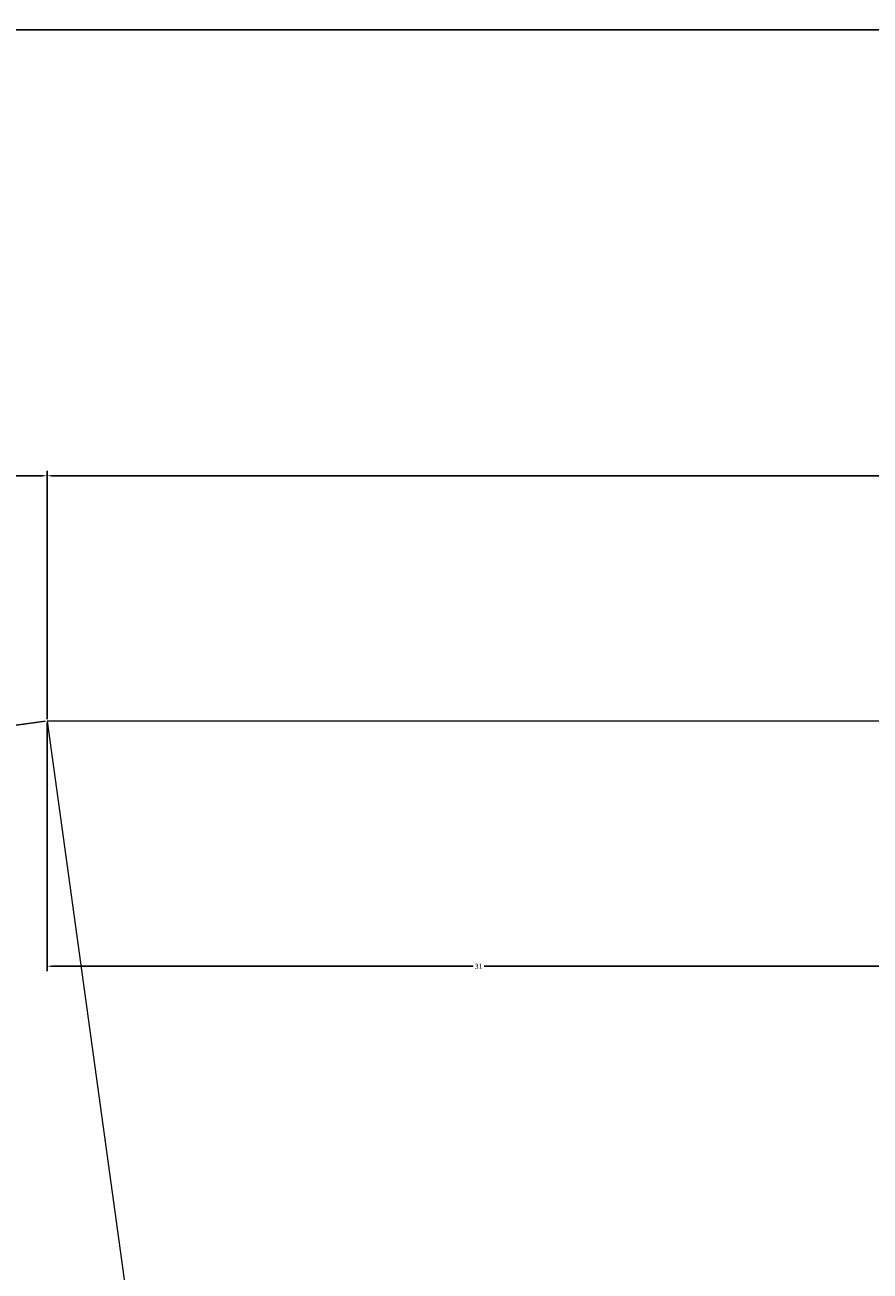
# Model space of a CAD drawing. Units: millimetres. Extents: x -9 to 135, y -119 to 27.
# Tile 5 of 12: x 31 to 62, y -18 to 27. Entities that reach past the tile are written whole.
import ezdxf

# ---------------------------------------------------------------- set-up
doc = ezdxf.new("R2010")
doc.units = ezdxf.units.MM
doc.layers.add('M-CONS', color=8, linetype='Continuous', lineweight=18)
doc.layers.add('M-DIMS', color=2, linetype='Continuous', lineweight=18)
doc.styles.get("Standard").update_dxf_attribs({"font": 'arial.ttf'})
doc.dimstyles.get("Standard").update_dxf_attribs({"dimtxt": 0.18, "dimasz": 0.18, "dimexe": 0.18, "dimexo": 0.0625, "dimgap": 0.09, "dimtad": 0, "dimtih": 1, "dimtoh": 1, "dimdec": 4, "dimzin": 0, "dimdsep": 46, "dimtxsty": 'Standard', "dimcen": 0.09, "dimadec": 0, "dimazin": 0, "dimtfac": 1, "dimtdec": 4, "dimtofl": 0, "dimtmove": 0, "dimatfit": 3, "dimfxl": 1, "dimtolj": 1, "dimtzin": 0, "dimarcsym": 0})

# ---------------------------------------------------------------- blocks, each defined once
blk = doc.blocks.new('*D2')
at = {"layer": 'Defpoints', "color": 0, "transparency": 16777216}
for p in [(126, 26.533), (0, 17.733), (126, 1.733)]:
    blk.add_point(p, dxfattribs=at)
at = {"layer": 'M-DIMS', "color": 0, "lineweight": -2, "transparency": 16777216}
for p, q in [((0, 17.796), (0, 26.713)), ((0.18, 26.533), (62.72, 26.533)), ((125.82, 26.533), (63.28, 26.533)), ((126, 1.796), (126, 26.713))]:
    blk.add_line(p, q, dxfattribs=at)
at = {"layer": 'M-DIMS', "color": 0, "transparency": 16777216}
for points in [[(0.18, 26.563), (0.18, 26.503), (0, 26.533)], [(125.82, 26.563), (125.82, 26.503), (126, 26.533)]]:
    blk.add_solid(points, dxfattribs=at)
at = {"layer": 'M-DIMS', "color": 0, "transparency": 16777216, "insert": (63, 26.533), "char_height": 0.18, "attachment_point": 5}
blk.add_mtext('\\A1;126', dxfattribs=at)
blk = doc.blocks.new('*D3')
at = {"layer": 'Defpoints', "color": 0, "transparency": 16777216}
for p in [(0, 17.733), (-8.8, -110.267), (63, -110.267)]:
    blk.add_point(p, dxfattribs=at)
at = {"layer": 'M-DIMS', "color": 0, "lineweight": -2, "transparency": 16777216}
for p, q in [((-0.062, 17.733), (-8.98, 17.733)), ((-8.8, 17.553), (-8.8, -46.085)), ((-8.8, -110.087), (-8.8, -46.449)), ((62.938, -110.267), (-8.98, -110.267))]:
    blk.add_line(p, q, dxfattribs=at)
at = {"layer": 'M-DIMS', "color": 0, "transparency": 16777216}
for points in [[(-8.83, 17.553), (-8.77, 17.553), (-8.8, 17.733)], [(-8.83, -110.087), (-8.77, -110.087), (-8.8, -110.267)]]:
    blk.add_solid(points, dxfattribs=at)
at = {"layer": 'M-DIMS', "color": 0, "transparency": 16777216, "insert": (-8.8, -46.267), "char_height": 0.18, "attachment_point": 5}
blk.add_mtext('\\A1;128', dxfattribs=at)
blk = doc.blocks.new('*D5')
at = {"layer": 'Defpoints', "color": 0, "transparency": 16777216}
for p in [(32, 10.533), (18, 1.733), (32, 1.733)]:
    blk.add_point(p, dxfattribs=at)
at = {"layer": 'M-DIMS', "color": 0, "lineweight": -2, "transparency": 16777216}
for p, q in [((18, 1.796), (18, 10.713)), ((18.18, 10.533), (24.79, 10.533)), ((31.82, 10.533), (25.21, 10.533)), ((32, 1.796), (32, 10.713))]:
    blk.add_line(p, q, dxfattribs=at)
at = {"layer": 'M-DIMS', "color": 0, "transparency": 16777216}
for points in [[(18.18, 10.563), (18.18, 10.503), (18, 10.533)], [(31.82, 10.563), (31.82, 10.503), (32, 10.533)]]:
    blk.add_solid(points, dxfattribs=at)
at = {"layer": 'M-DIMS', "color": 0, "transparency": 16777216, "insert": (25, 10.533), "char_height": 0.18, "attachment_point": 5}
blk.add_mtext('\\A1;14', dxfattribs=at)
blk = doc.blocks.new('*D6')
at = {"layer": 'Defpoints', "color": 0, "transparency": 16777216}
for p in [(94, 10.533), (32, 1.733), (94, 1.733)]:
    blk.add_point(p, dxfattribs=at)
at = {"layer": 'M-DIMS', "color": 0, "lineweight": -2, "transparency": 16777216}
for p, q in [((32, 1.796), (32, 10.713)), ((32.18, 10.533), (62.782, 10.533)), ((93.82, 10.533), (63.218, 10.533)), ((94, 1.796), (94, 10.713))]:
    blk.add_line(p, q, dxfattribs=at)
at = {"layer": 'M-DIMS', "color": 0, "transparency": 16777216}
for points in [[(32.18, 10.563), (32.18, 10.503), (32, 10.533)], [(93.82, 10.563), (93.82, 10.503), (94, 10.533)]]:
    blk.add_solid(points, dxfattribs=at)
at = {"layer": 'M-DIMS', "color": 0, "transparency": 16777216, "insert": (63, 10.533), "char_height": 0.18, "attachment_point": 5}
blk.add_mtext('\\A1;62', dxfattribs=at)
blk = doc.blocks.new('*D9')
at = {"layer": 'Defpoints', "color": 0, "transparency": 16777216}
for p in [(32, 1.733), (63, 1.733), (32, -7.067)]:
    blk.add_point(p, dxfattribs=at)
at = {"layer": 'M-DIMS', "color": 0, "lineweight": -2, "transparency": 16777216}
for p, q in [((32, 1.671), (32, -7.247)), ((63, 1.671), (63, -7.247)), ((32.18, -7.067), (47.299, -7.067)), ((62.82, -7.067), (47.701, -7.067))]:
    blk.add_line(p, q, dxfattribs=at)
at = {"layer": 'M-DIMS', "color": 0, "transparency": 16777216}
for points in [[(32.18, -7.037), (32.18, -7.097), (32, -7.067)], [(62.82, -7.037), (62.82, -7.097), (63, -7.067)]]:
    blk.add_solid(points, dxfattribs=at)
at = {"layer": 'M-DIMS', "color": 0, "transparency": 16777216, "insert": (47.5, -7.067), "char_height": 0.18, "attachment_point": 5}
blk.add_mtext('\\A1;31', dxfattribs=at)
blk = doc.blocks.new('*D14')
at = {"layer": 'Defpoints', "color": 0, "transparency": 16777216}
for p in [(32, 1.733), (23.283, 0.528), (45, -92.267)]:
    blk.add_point(p, dxfattribs=at)
at = {"layer": 'M-DIMS', "color": 0, "lineweight": -2, "transparency": 16777216}
for p, q in [((31.938, 1.725), (23.105, 0.503)), ((23.308, 0.349), (29.758, -46.29)), ((36.258, -93.294), (29.808, -46.654)), ((44.938, -92.275), (36.105, -93.497))]:
    blk.add_line(p, q, dxfattribs=at)
at = {"layer": 'M-DIMS', "color": 0, "transparency": 16777216}
for points in [[(23.337, 0.353), (23.278, 0.345), (23.283, 0.528)], [(36.288, -93.29), (36.229, -93.298), (36.283, -93.472)]]:
    blk.add_solid(points, dxfattribs=at)
at = {"layer": 'M-DIMS', "color": 0, "transparency": 16777216, "insert": (29.783, -46.472), "char_height": 0.18, "attachment_point": 5}
blk.add_mtext('\\A1;94.9', dxfattribs=at)

msp = doc.modelspace()

# ---------------------------------------------------------------- linework, layer by layer
at = {"layer": 'M-CONS'}
for p, q in [((63, 1.733, 115.129), (32, 1.733, 115.129)), ((32, 1.733, 115.129), (45, -92.267, 115.129))]:
    msp.add_line(p, q, dxfattribs=at)

# ---------------------------------------------------------------- dimensions: what is measured, and where the dimension line sits
at = {"layer": 'M-DIMS'}
for base, p1, p2, picture, middle in [((126, 26.533), (0, 17.733), (126, 1.733), '*D2', (63, 26.533)), ((32, 10.533), (18, 1.733), (32, 1.733), '*D5', (25, 10.533)), ((94, 10.533), (32, 1.733), (94, 1.733), '*D6', (63, 10.533))]:
    dim = msp.add_linear_dim(base=base, p1=p1, p2=p2, dimstyle='Standard', override={"dimdec": 0, "dimlfac": 1, "dimrnd": 0, "dimzin": 0, "dimdsep": 46, "dimlunit": 2}, dxfattribs=at)
    dim.commit()
    dim.dimension.update_dxf_attribs({"geometry": picture, "text_midpoint": middle})
for base, p1, p2, angle, override, picture, middle in [((-8.8, -110.267), (0, 17.733), (63, -110.267), 90, {"dimdec": 0, "dimlfac": 1, "dimrnd": 0, "dimzin": 0, "dimdsep": 46, "dimlunit": 2}, '*D3', (-8.8, -46.267)), ((23.283, 0.528), (45, -92.267), (32, 1.733), 97.8739, {"dimdec": 1, "dimlfac": 1, "dimrnd": 0, "dimzin": 0, "dimdsep": 46, "dimlunit": 2}, '*D14', (29.783, -46.472)), ((32, -7.067), (63, 1.733), (32, 1.733), 180, {"dimdec": 0, "dimlfac": 1, "dimrnd": 0, "dimzin": 0, "dimdsep": 46, "dimlunit": 2}, '*D9', (47.5, -7.067))]:
    dim = msp.add_linear_dim(base=base, p1=p1, p2=p2, angle=angle, dimstyle='Standard', override=override, dxfattribs=at)
    dim.commit()
    dim.dimension.update_dxf_attribs({"geometry": picture, "text_midpoint": middle})

doc.saveas('drawing.dxf')
